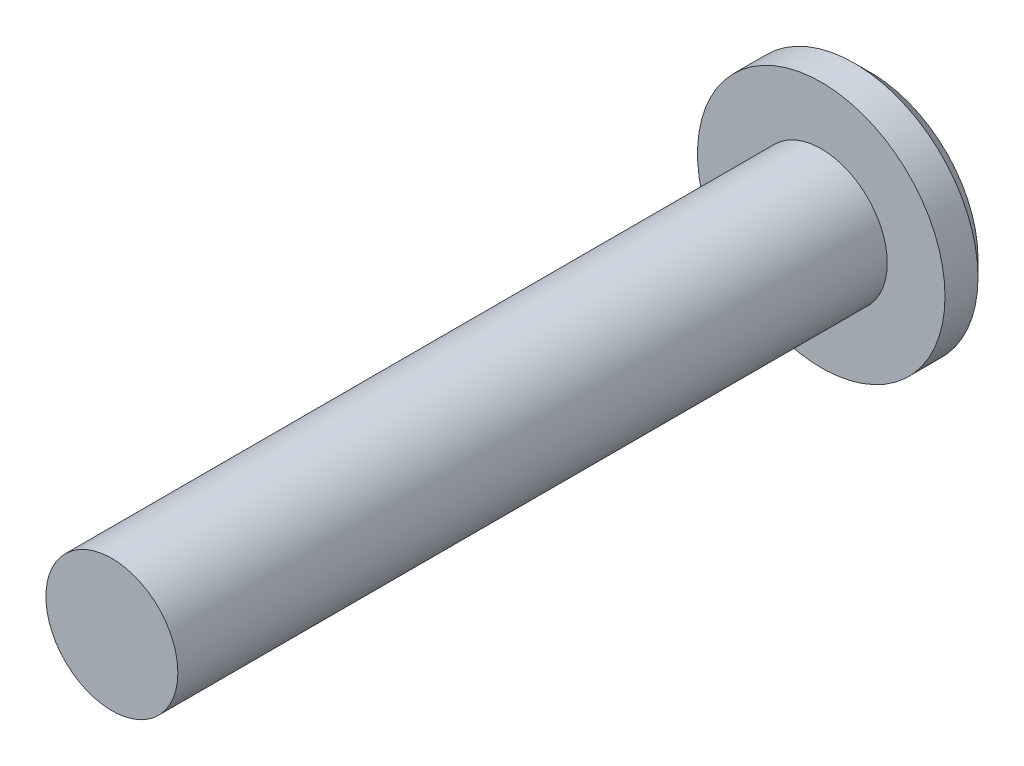
ISO-10303-21;
HEADER;
FILE_DESCRIPTION(('STEP AP214'),'2;1');
FILE_NAME('part.step','',(''),(''),'','','');
FILE_SCHEMA(('AUTOMOTIVE_DESIGN { 1 0 10303 214 1 1 1 1 }'));
ENDSEC;
DATA;
#1=APPLICATION_CONTEXT('core data for automotive mechanical design processes');
#2=APPLICATION_PROTOCOL_DEFINITION('international standard','automotive_design',2000,#1);
#3=PRODUCT_CONTEXT('',#1,'mechanical');
#4=PRODUCT('Part','Part','',(#3));
#5=PRODUCT_RELATED_PRODUCT_CATEGORY('part','',(#4));
#6=PRODUCT_DEFINITION_FORMATION('','',#4);
#7=PRODUCT_DEFINITION_CONTEXT('part definition',#1,'design');
#8=PRODUCT_DEFINITION('design','',#6,#7);
#9=PRODUCT_DEFINITION_SHAPE('','',#8);
#10=(LENGTH_UNIT() NAMED_UNIT(*) SI_UNIT(.MILLI.,.METRE.));
#11=(NAMED_UNIT(*) PLANE_ANGLE_UNIT() SI_UNIT($,.RADIAN.));
#12=(NAMED_UNIT(*) SI_UNIT($,.STERADIAN.) SOLID_ANGLE_UNIT());
#13=UNCERTAINTY_MEASURE_WITH_UNIT(LENGTH_MEASURE(1.E-05),#10,'distance_accuracy_value','');
#14=(GEOMETRIC_REPRESENTATION_CONTEXT(3) GLOBAL_UNCERTAINTY_ASSIGNED_CONTEXT((#13)) GLOBAL_UNIT_ASSIGNED_CONTEXT((#10,
#11,#12)) REPRESENTATION_CONTEXT('',''));
#15=CARTESIAN_POINT('',(0.,0.,0.));
#16=DIRECTION('',(0.,0.,1.));
#17=DIRECTION('',(1.,0.,0.));
#18=AXIS2_PLACEMENT_3D('',#15,#16,#17);
#19=CARTESIAN_POINT('',(0.,0.,3.));
#20=DIRECTION('',(0.,0.,-1.));
#21=DIRECTION('',(-1.,0.,0.));
#22=AXIS2_PLACEMENT_3D('',#19,#20,#21);
#23=CYLINDRICAL_SURFACE('',#22,7.5);
#24=CARTESIAN_POINT('',(0.,0.,1.00000000000001));
#25=DIRECTION('',(0.,0.,1.));
#26=DIRECTION('',(1.,0.,0.));
#27=AXIS2_PLACEMENT_3D('',#24,#25,#26);
#28=CIRCLE('',#27,7.5);
#29=CARTESIAN_POINT('',(7.5,0.,1.00000000000001));
#30=VERTEX_POINT('',#29);
#31=EDGE_CURVE('E52',#30,#30,#28,.T.);
#32=ORIENTED_EDGE('',*,*,#31,.T.);
#33=EDGE_LOOP('',(#32));
#34=FACE_BOUND('',#33,.T.);
#35=CARTESIAN_POINT('',(0.,0.,3.));
#36=DIRECTION('',(0.,0.,1.));
#37=DIRECTION('',(1.,0.,0.));
#38=AXIS2_PLACEMENT_3D('',#35,#36,#37);
#39=CIRCLE('',#38,7.5);
#40=CARTESIAN_POINT('',(7.5,0.,3.));
#41=VERTEX_POINT('',#40);
#42=EDGE_CURVE('E61',#41,#41,#39,.T.);
#43=ORIENTED_EDGE('',*,*,#42,.F.);
#44=EDGE_LOOP('',(#43));
#45=FACE_BOUND('',#44,.T.);
#46=ADVANCED_FACE('F44',(#34,#45),#23,.T.);
#47=CARTESIAN_POINT('',(0.,0.,3.));
#48=DIRECTION('',(0.,0.,1.));
#49=DIRECTION('',(1.,0.,0.));
#50=AXIS2_PLACEMENT_3D('',#47,#48,#49);
#51=PLANE('',#50);
#52=CARTESIAN_POINT('',(0.,0.,3.));
#53=DIRECTION('',(0.,0.,1.));
#54=DIRECTION('',(1.,0.,0.));
#55=AXIS2_PLACEMENT_3D('',#52,#53,#54);
#56=CIRCLE('',#55,4.);
#57=CARTESIAN_POINT('',(4.,0.,3.));
#58=VERTEX_POINT('',#57);
#59=EDGE_CURVE('E60',#58,#58,#56,.T.);
#60=ORIENTED_EDGE('',*,*,#59,.F.);
#61=EDGE_LOOP('',(#60));
#62=FACE_BOUND('',#61,.T.);
#63=ORIENTED_EDGE('',*,*,#42,.T.);
#64=EDGE_LOOP('',(#63));
#65=FACE_BOUND('',#64,.T.);
#66=ADVANCED_FACE('F78',(#62,#65),#51,.T.);
#67=CARTESIAN_POINT('',(0.,0.,0.));
#68=DIRECTION('',(0.,0.,1.));
#69=DIRECTION('',(1.,0.,0.));
#70=AXIS2_PLACEMENT_3D('',#67,#68,#69);
#71=PLANE('',#70);
#72=CARTESIAN_POINT('',(0.,0.,0.));
#73=DIRECTION('',(0.,0.,1.));
#74=DIRECTION('',(1.,0.,0.));
#75=AXIS2_PLACEMENT_3D('',#72,#73,#74);
#76=CIRCLE('',#75,6.49999999999999);
#77=CARTESIAN_POINT('',(6.49999999999999,0.,0.));
#78=VERTEX_POINT('',#77);
#79=EDGE_CURVE('E10',#78,#78,#76,.F.);
#80=ORIENTED_EDGE('',*,*,#79,.T.);
#81=EDGE_LOOP('',(#80));
#82=FACE_BOUND('',#81,.T.);
#83=ADVANCED_FACE('F73',(#82),#71,.F.);
#84=CARTESIAN_POINT('',(0.,0.,46.));
#85=DIRECTION('',(0.,0.,-1.));
#86=DIRECTION('',(-1.,0.,0.));
#87=AXIS2_PLACEMENT_3D('',#84,#85,#86);
#88=CYLINDRICAL_SURFACE('',#87,4.);
#89=CARTESIAN_POINT('',(0.,0.,46.));
#90=DIRECTION('',(0.,0.,1.));
#91=DIRECTION('',(1.,0.,0.));
#92=AXIS2_PLACEMENT_3D('',#89,#90,#91);
#93=CIRCLE('',#92,4.);
#94=CARTESIAN_POINT('',(4.,0.,46.));
#95=VERTEX_POINT('',#94);
#96=EDGE_CURVE('E64',#95,#95,#93,.T.);
#97=ORIENTED_EDGE('',*,*,#96,.F.);
#98=EDGE_LOOP('',(#97));
#99=FACE_BOUND('',#98,.T.);
#100=ORIENTED_EDGE('',*,*,#59,.T.);
#101=EDGE_LOOP('',(#100));
#102=FACE_BOUND('',#101,.T.);
#103=ADVANCED_FACE('F75',(#99,#102),#88,.T.);
#104=CARTESIAN_POINT('',(0.,0.,46.));
#105=DIRECTION('',(0.,0.,1.));
#106=DIRECTION('',(1.,0.,0.));
#107=AXIS2_PLACEMENT_3D('',#104,#105,#106);
#108=PLANE('',#107);
#109=ORIENTED_EDGE('',*,*,#96,.T.);
#110=EDGE_LOOP('',(#109));
#111=FACE_BOUND('',#110,.T.);
#112=ADVANCED_FACE('F69',(#111),#108,.T.);
#113=CARTESIAN_POINT('',(0.,0.,1.00000000000001));
#114=DIRECTION('',(0.,0.,1.));
#115=DIRECTION('',(1.,0.,0.));
#116=AXIS2_PLACEMENT_3D('',#113,#114,#115);
#117=CONICAL_SURFACE('',#116,7.5,0.78539816339745);
#118=ORIENTED_EDGE('',*,*,#79,.F.);
#119=EDGE_LOOP('',(#118));
#120=FACE_BOUND('',#119,.T.);
#121=ORIENTED_EDGE('',*,*,#31,.F.);
#122=EDGE_LOOP('',(#121));
#123=FACE_BOUND('',#122,.T.);
#124=ADVANCED_FACE('F48',(#120,#123),#117,.T.);
#125=CLOSED_SHELL('',(#46,#66,#83,#103,#112,#124));
#126=MANIFOLD_SOLID_BREP('B2',#125);
#127=ADVANCED_BREP_SHAPE_REPRESENTATION('',(#18,#126),#14);
#128=SHAPE_DEFINITION_REPRESENTATION(#9,#127);
ENDSEC;
END-ISO-10303-21;
